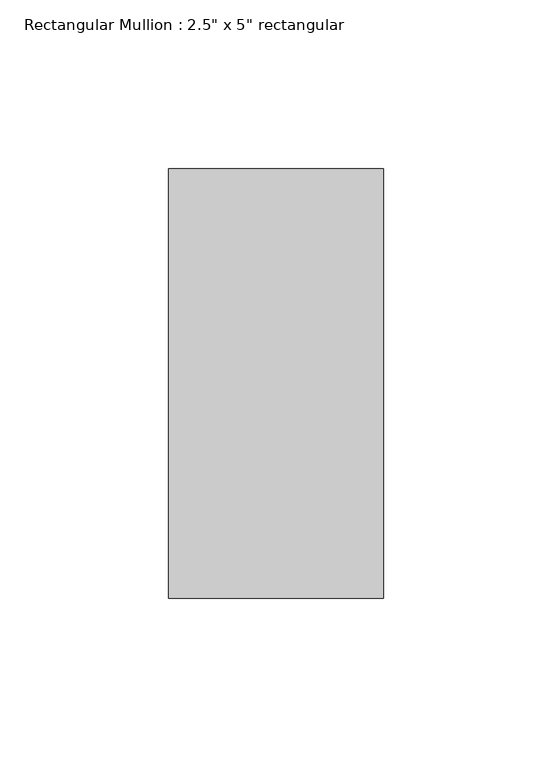
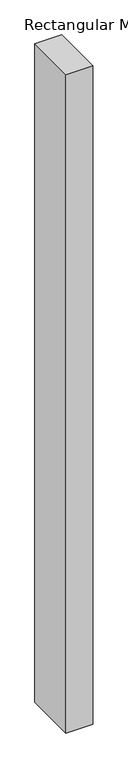
"""IFC4 building model written with IfcOpenShell, lengths in millimetres: member geometry."""

from ifc_helpers import new_model, si_unit, frame, origin, place, context, project, spatial, polyline, outline, extrude, source, transform, mapped, element, save


def member_dca25542(model_context):
    return source(origin(), model_context, "Body", "SweptSolid", [
        extrude(outline(polyline([(0.0, 63.5), (0.0, -63.5), (-63.5, -63.5), (-63.5, 63.5), (0.0, 63.5)])), frame((0.0, 0.0, -1644.3056511), z_axis=(0.0, 0.0, 1.0), x_axis=(1.0, 0.0, 0.0)), (0.0, 0.0, 1.0), 1644.3056511),
    ])


if __name__ == "__main__":
    model = new_model("IFC4")
    model_context = context("Model", 3, world=origin())
    ifc_project = project(units=[si_unit("LENGTHUNIT", "METRE", prefix="MILLI")], contexts=[model_context])
    site = spatial("IfcSite", under=ifc_project)
    building = spatial("IfcBuilding", under=site)
    placement = place(None, origin())
    member_shape = member_dca25542(model_context)
    element("IfcMember", 1, ObjectType="Rectangular Mullion : 2.5\" x 5\" rectangular", at=placement, inside=building, context=model_context, shape_type="MappedRepresentation", body=[
        mapped(member_shape, transform((0.0, 0.0, 0.0), x_axis=(1.0, 0.0, 0.0), y_axis=(0.0, 1.0, 0.0), z_axis=(0.0, 0.0, 1.0))),
    ])
    save(model, "model.ifc")

# Revit data of these elements
# Type "Rectangular Mullion : 2.5\" x 5\" rectangular"
#   built-in parameter 1007304 = 0.416667 (stored number, unit not read)
#   built-in parameter 1007301 = 0.104167 (stored number, unit not read)
#   built-in parameter 1007300 = 0.104167 (stored number, unit not read)
# Element 1 (IfcMember, "Rectangular Mullion : 2.5\" x 5\" rectangular")
#   Materials on its faces: "Aluminum"
# Materials
#   "Aluminum": class "Metal", colour RGB 247 247 247, transparency 0, Description = "Aluminum 6061", Cost = 0
